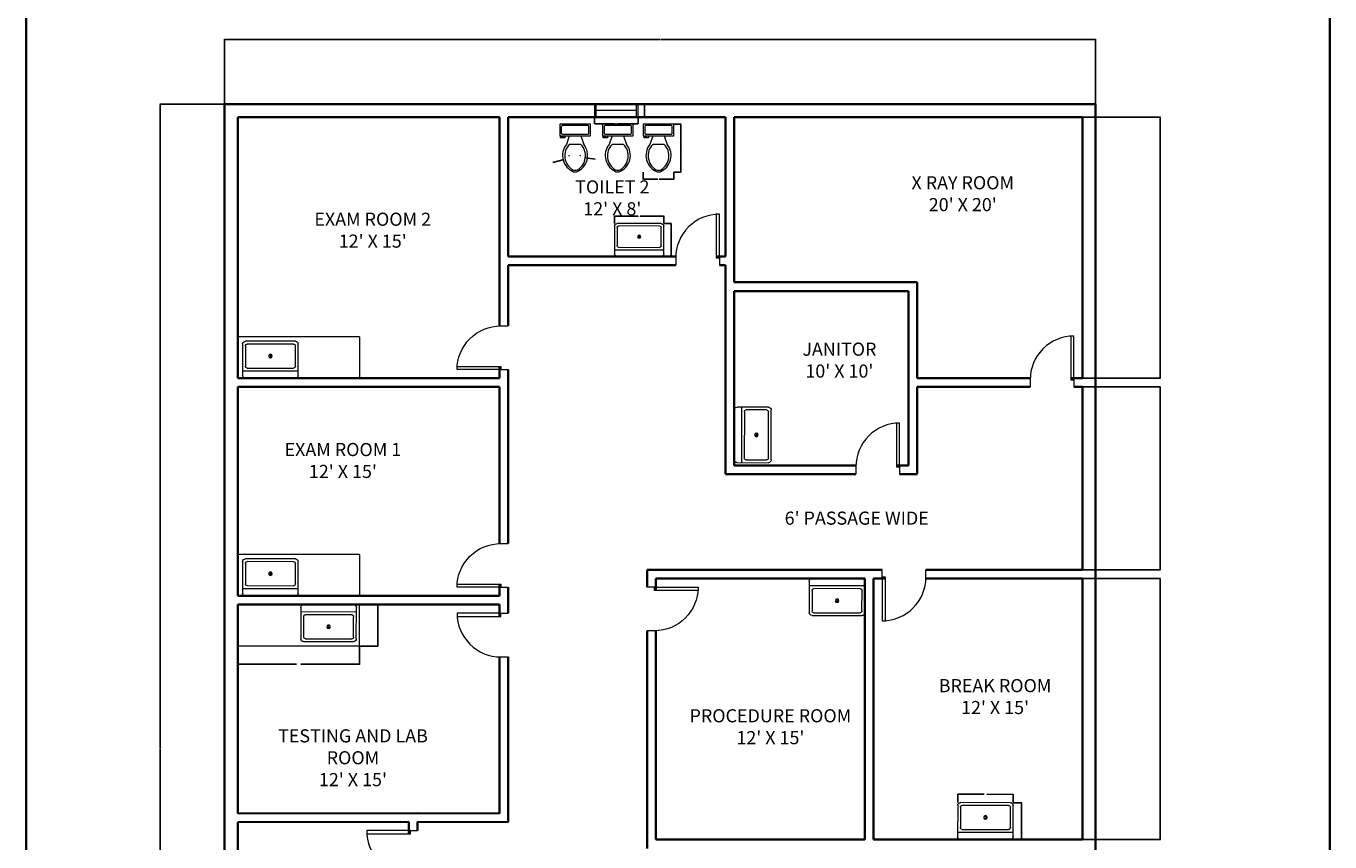
# Model space of a CAD drawing. Units: inches. Extents: x 7245 to 8143, y 15548 to 17244.
# Tile 4 of 5: x 7245 to 8143, y 16334 to 16896. Entities that reach past the tile are written whole.
import ezdxf

# ---------------------------------------------------------------- set-up
doc = ezdxf.new("R2010")
doc.units = ezdxf.units.IN
for name, color, linetype, lineweight in [('A-ANNO-DIMS', 2, 'Continuous', 18), ('A-ANNO-TTLB', 7, 'Continuous', 35), ('A-AREA-IDEN', 7, 'Continuous', 18), ('A-DOOR', 3, 'Continuous', 18), ('A-FLOR-CASE', 9, 'Continuous', 20), ('A-FLOR-FIXT', 9, 'Continuous', 18), ('A-GLAZ', 4, 'Continuous', 18), ('A-WALL', 7, 'Continuous', 35)]:
    doc.layers.add(name, color=color, linetype=linetype, lineweight=lineweight)
doc.styles.get("Standard").update_dxf_attribs({"font": 'arial.ttf'})
doc.dimstyles.get("Standard").update_dxf_attribs({"dimtxt": 0.18, "dimasz": 0.18, "dimexe": 0.18, "dimexo": 0.0625, "dimgap": 0.09, "dimtad": 0, "dimtih": 1, "dimtoh": 1, "dimdec": 4, "dimzin": 0, "dimdsep": 46, "dimtxsty": 'Standard', "dimcen": 0.09, "dimadec": 0, "dimazin": 0, "dimtfac": 1, "dimtdec": 4, "dimtofl": 0, "dimtmove": 0, "dimatfit": 3, "dimfxl": 1, "dimtolj": 1, "dimtzin": 0, "dimarcsym": 0})

# ---------------------------------------------------------------- blocks, each defined once
blk = doc.blocks.new('Sink-single - 30 in top')
blk.add_line((-15, -3.999996), (15, -3.999996))
for points in [[(-13.5, 0), (13.5, 0)], [(-15, -18.499996), (-15, -1.5)], [(-13.5, -17.499996), (-13.5, -6.499996)], [(-12.5, -5.499996), (12.5, -5.499996)], [(13.5, -6.499996), (13.5, -17.499996)], [(15, -1.5), (15, -18.499996)], [(13.5, -19.999996), (-13.5, -19.999996)], [(12.5, -18.499996), (-12.5, -18.499996)]]:
    blk.add_lwpolyline(points)
for radius in [1, 0.5]:
    blk.add_circle((0, -11.999996), radius)
for centre, radius, start, end in [((-13.5, -1.5), 1.5, 90, 180), ((-12.5, -6.499996), 1, 90, 180), ((12.5, -6.499996), 1, 0, 90), ((13.5, -1.5), 1.5, 0, 90), ((-13.5, -18.499996), 1.5, 180, 270), ((-12.5, -17.499996), 1, 180, 270), ((12.5, -17.499996), 1, 270, 0), ((13.5, -18.499996), 1.5, 270, 0)]:
    blk.add_arc(centre, radius, start, end)
blk = doc.blocks.new('*U9')
for p, q in [((0, 0), (0, 100)), ((600, 0), (600, 100))]:
    blk.add_line(p, q)
blk.add_lwpolyline([(0, 0), (0, -600), (43.75, -600), (43.75, 0)], close=True)
blk.add_arc((0, 0), 600, 270, 0)
blk = doc.blocks.new('Toilet - top')
for p, q in [((-10, -8.5), (-8, -8.5)), ((-10, -9.5), (-10, -8.5)), ((-8, -8.5), (-8, -8)), ((-7, -8), (-7, -9.5)), ((-4, -8), (-6, -14)), ((4, -8), (6, -14)), ((9.5, -6), (9.5, -2)), ((-7, -9.5), (-10, -9.5)), ((4, -14), (-4, -14))]:
    blk.add_line(p, q)
blk.add_lwpolyline([(10.5, -8), (10.5, 0), (-10.5, 0), (-10.5, -8)], close=True)
for points in [[(-9.5, -2), (-9.5, -6)], [(8.5, -1), (-8.5, -1)], [(-8.5, -7), (8.5, -7)]]:
    blk.add_lwpolyline(points)
for centre, radius, start, end in [((-8.62, -1.88), 0.884, 81.8699, 188.1301), ((-8.62, -6.12), 0.884, 171.8699, 278.1301), ((8.62, -1.88), 0.884, 351.8699, 98.1301), ((8.62, -6.12), 0.884, 261.8699, 8.1301), ((3.52, -21.58), 12.17, 141.46911, 247.97143), ((4.2, -21.82), 11.33, 136.36773, 238.94682), ((-3.52, -21.58), 12.17, 292.02843, 38.53071), ((-4.2, -21.82), 11.33, 301.05301, 43.63209), ((0, -27.88), 4, 245.73182, 294.26817), ((0, -29), 4, 254.86053, 285.13947)]:
    blk.add_arc(centre, radius, start, end)
blk = doc.blocks.new('WINDOW-30IN-PLAN')
for p, q in [((30, 9), (0, 9)), ((0, 9), (0, 0)), ((1, 9), (1, 0)), ((29, 0), (29, 9)), ((30, 0), (30, 9)), ((29, 4.5), (1, 4.5)), ((0, 0), (30, 0))]:
    blk.add_line(p, q)
blk = doc.blocks.new('SINK-COUNTER-84IN')
for q in [(84, 28.58), (0, 0)]:
    blk.add_line((84, 0), q)
blk = doc.blocks.new('*D20')
at = {"layer": 'A-ANNO-DIMS', "color": 0, "lineweight": -2, "transparency": 16777216}
for p, q in [((7887.06, 16360.81), (7887.08, 16366.67)), ((7887.26, 16366.49), (7905.26, 16366.45)), ((7925.14, 16366.4), (7907.13, 16366.44)), ((7925.31, 16360.73), (7925.32, 16366.58))]:
    blk.add_line(p, q, dxfattribs=at)
at = {"layer": 'A-ANNO-DIMS', "color": 0, "transparency": 16777216}
for points in [[(7887.26, 16366.52), (7887.26, 16366.46), (7887.08, 16366.49)], [(7925.14, 16366.43), (7925.14, 16366.37), (7925.32, 16366.4)]]:
    blk.add_solid(points, dxfattribs=at)
at = {"layer": 'Defpoints', "color": 0, "transparency": 16777216}
for p in [(7925.32, 16366.4), (7887.06, 16360.75), (7925.31, 16360.67)]:
    blk.add_point(p, dxfattribs=at)
at = {"layer": 'A-ANNO-DIMS', "color": 0, "transparency": 16777216, "insert": (7906.2, 16366.44), "char_height": 0.18, "attachment_point": 5}
blk.add_mtext('\\A1;BASIN 38 TYP.', dxfattribs=at)
blk = doc.blocks.new('*D21')
at = {"layer": 'A-ANNO-DIMS', "color": 0, "lineweight": -2, "transparency": 16777216}
for p, q in [((7925.37, 16360.67), (7931.22, 16360.65)), ((7931.04, 16360.48), (7931.02, 16348.09)), ((7930.99, 16335.34), (7931.01, 16347.73)), ((7925.31, 16335.17), (7931.17, 16335.16))]:
    blk.add_line(p, q, dxfattribs=at)
at = {"layer": 'A-ANNO-DIMS', "color": 0, "transparency": 16777216}
for points in [[(7931.01, 16360.48), (7931.07, 16360.48), (7931.04, 16360.66)], [(7930.96, 16335.34), (7931.02, 16335.34), (7930.99, 16335.16)]]:
    blk.add_solid(points, dxfattribs=at)
at = {"layer": 'Defpoints', "color": 0, "transparency": 16777216}
for p in [(7925.31, 16360.67), (7925.25, 16335.17), (7930.99, 16335.16)]:
    blk.add_point(p, dxfattribs=at)
at = {"layer": 'A-ANNO-DIMS', "color": 0, "transparency": 16777216, "insert": (7931.02, 16347.91), "char_height": 0.18, "attachment_point": 5}
blk.add_mtext('\\A1;25 TYP.', dxfattribs=at)
blk = doc.blocks.new('*D22')
at = {"layer": 'A-ANNO-DIMS', "color": 0, "lineweight": -2, "transparency": 16777216}
for p, q in [((7650.71, 16759.93), (7650.72, 16765.13)), ((7650.9, 16764.95), (7667.03, 16764.92)), ((7684.42, 16764.88), (7668.29, 16764.91)), ((7684.59, 16759.86), (7684.6, 16765.06))]:
    blk.add_line(p, q, dxfattribs=at)
at = {"layer": 'A-ANNO-DIMS', "color": 0, "transparency": 16777216}
for points in [[(7650.9, 16764.98), (7650.9, 16764.92), (7650.72, 16764.95)], [(7684.42, 16764.91), (7684.42, 16764.85), (7684.6, 16764.88)]]:
    blk.add_solid(points, dxfattribs=at)
at = {"layer": 'Defpoints', "color": 0, "transparency": 16777216}
for p in [(7684.6, 16764.88), (7650.71, 16759.87), (7684.59, 16759.8)]:
    blk.add_point(p, dxfattribs=at)
at = {"layer": 'A-ANNO-DIMS', "color": 0, "transparency": 16777216, "insert": (7667.66, 16764.92), "char_height": 0.18, "attachment_point": 5}
blk.add_mtext('\\A1;BASIN 34', dxfattribs=at)
blk = doc.blocks.new('*D23')
at = {"layer": 'A-ANNO-DIMS', "color": 0, "lineweight": -2, "transparency": 16777216}
for p, q in [((7684.65, 16759.8), (7689.85, 16759.79)), ((7689.67, 16759.61), (7689.65, 16748.67)), ((7689.62, 16737.38), (7689.65, 16748.31)), ((7684.6, 16737.21), (7689.8, 16737.2))]:
    blk.add_line(p, q, dxfattribs=at)
at = {"layer": 'A-ANNO-DIMS', "color": 0, "transparency": 16777216}
for points in [[(7689.64, 16759.61), (7689.7, 16759.61), (7689.67, 16759.79)], [(7689.59, 16737.38), (7689.65, 16737.38), (7689.62, 16737.2)]]:
    blk.add_solid(points, dxfattribs=at)
at = {"layer": 'Defpoints', "color": 0, "transparency": 16777216}
for p in [(7684.59, 16759.8), (7684.54, 16737.21), (7689.62, 16737.2)]:
    blk.add_point(p, dxfattribs=at)
at = {"layer": 'A-ANNO-DIMS', "color": 0, "transparency": 16777216, "insert": (7689.65, 16748.49), "char_height": 0.18, "attachment_point": 5}
blk.add_mtext('\\A1;23', dxfattribs=at)
blk = doc.blocks.new('*D30')
at = {"layer": 'A-ANNO-DIMS', "color": 0, "lineweight": -2, "transparency": 16777216}
for p, q in [((7691.53, 16828.41), (7696.61, 16828.41)), ((7696.43, 16828.23), (7696.43, 16812.07)), ((7696.43, 16795.54), (7696.43, 16811.7)), ((7691.53, 16795.36), (7696.61, 16795.36))]:
    blk.add_line(p, q, dxfattribs=at)
at = {"layer": 'A-ANNO-DIMS', "color": 0, "transparency": 16777216}
for points in [[(7696.4, 16828.23), (7696.46, 16828.23), (7696.43, 16828.41)], [(7696.4, 16795.54), (7696.46, 16795.54), (7696.43, 16795.36)]]:
    blk.add_solid(points, dxfattribs=at)
at = {"layer": 'Defpoints', "color": 0, "transparency": 16777216}
for p in [(7691.47, 16828.41), (7696.43, 16828.41), (7691.47, 16795.36)]:
    blk.add_point(p, dxfattribs=at)
at = {"layer": 'A-ANNO-DIMS', "color": 0, "transparency": 16777216, "insert": (7696.43, 16811.89), "char_height": 0.18, "attachment_point": 5}
blk.add_mtext('\\A1;WC 33 TYP.', dxfattribs=at)
blk = doc.blocks.new('*D31')
at = {"layer": 'A-ANNO-DIMS', "color": 0, "lineweight": -2, "transparency": 16777216}
for p, q in [((7670.47, 16795.3), (7670.47, 16790.23)), ((7670.65, 16790.41), (7680.44, 16790.41)), ((7691.29, 16790.41), (7681.5, 16790.41)), ((7691.47, 16795.3), (7691.47, 16790.23))]:
    blk.add_line(p, q, dxfattribs=at)
at = {"layer": 'A-ANNO-DIMS', "color": 0, "transparency": 16777216}
for points in [[(7670.65, 16790.44), (7670.65, 16790.38), (7670.47, 16790.41)], [(7691.29, 16790.44), (7691.29, 16790.38), (7691.47, 16790.41)]]:
    blk.add_solid(points, dxfattribs=at)
at = {"layer": 'Defpoints', "color": 0, "transparency": 16777216}
for p in [(7670.47, 16795.36), (7691.47, 16795.36), (7691.47, 16790.41)]:
    blk.add_point(p, dxfattribs=at)
at = {"layer": 'A-ANNO-DIMS', "color": 0, "transparency": 16777216, "insert": (7680.97, 16790.41), "char_height": 0.18, "attachment_point": 5}
blk.add_mtext('\\A1;21 TYP.', dxfattribs=at)
blk = doc.blocks.new('*D32')
at = {"layer": 'A-ANNO-DIMS', "color": 0, "lineweight": -2, "transparency": 16777216}
for p, q in [((7391.08, 16468.57), (7391.08, 16455.85)), ((7475.08, 16468.57), (7475.08, 16455.85)), ((7391.26, 16456.03), (7431.57, 16456.03)), ((7474.9, 16456.03), (7434.6, 16456.03))]:
    blk.add_line(p, q, dxfattribs=at)
at = {"layer": 'A-ANNO-DIMS', "color": 0, "transparency": 16777216}
for points in [[(7391.26, 16456.06), (7391.26, 16456), (7391.08, 16456.03)], [(7474.9, 16456.06), (7474.9, 16456), (7475.08, 16456.03)]]:
    blk.add_solid(points, dxfattribs=at)
at = {"layer": 'Defpoints', "color": 0, "transparency": 16777216}
for p in [(7391.08, 16468.63), (7475.08, 16468.63), (7475.08, 16456.03)]:
    blk.add_point(p, dxfattribs=at)
at = {"layer": 'A-ANNO-DIMS', "color": 0, "transparency": 16777216, "insert": (7433.08, 16456.03), "char_height": 0.18, "attachment_point": 5}
blk.add_mtext('\\A1;SINK COUNTER 84 TYP.', dxfattribs=at)
blk = doc.blocks.new('*D33')
at = {"layer": 'A-ANNO-DIMS', "color": 0, "lineweight": -2, "transparency": 16777216}
for p, q in [((7475.15, 16497.21), (7487.86, 16497.21)), ((7487.68, 16497.03), (7487.68, 16483.11)), ((7487.68, 16468.81), (7487.68, 16482.74)), ((7475.15, 16468.63), (7487.86, 16468.63))]:
    blk.add_line(p, q, dxfattribs=at)
at = {"layer": 'A-ANNO-DIMS', "color": 0, "transparency": 16777216}
for points in [[(7487.65, 16497.03), (7487.71, 16497.03), (7487.68, 16497.21)], [(7487.65, 16468.81), (7487.71, 16468.81), (7487.68, 16468.63)]]:
    blk.add_solid(points, dxfattribs=at)
at = {"layer": 'Defpoints', "color": 0, "transparency": 16777216}
for p in [(7475.08, 16497.21), (7487.68, 16497.21), (7475.08, 16468.63)]:
    blk.add_point(p, dxfattribs=at)
at = {"layer": 'A-ANNO-DIMS', "color": 0, "transparency": 16777216, "insert": (7487.68, 16482.92), "char_height": 0.18, "attachment_point": 5}
blk.add_mtext('\\A1;29 TYP.', dxfattribs=at)
blk = doc.blocks.new('*D36')
at = {"layer": 'A-ANNO-DIMS', "color": 0, "lineweight": -2, "transparency": 16777216}
for p, q in [((7636.84, 16833.13), (7636.84, 16828.51)), ((7666.84, 16833.13), (7666.84, 16828.51)), ((7637.02, 16828.69), (7650.72, 16828.69)), ((7666.66, 16828.69), (7652.96, 16828.69))]:
    blk.add_line(p, q, dxfattribs=at)
at = {"layer": 'A-ANNO-DIMS', "color": 0, "transparency": 16777216}
for points in [[(7637.02, 16828.72), (7637.02, 16828.66), (7636.84, 16828.69)], [(7666.66, 16828.72), (7666.66, 16828.66), (7666.84, 16828.69)]]:
    blk.add_solid(points, dxfattribs=at)
at = {"layer": 'Defpoints', "color": 0, "transparency": 16777216}
for p in [(7636.84, 16833.19), (7666.84, 16833.19), (7666.84, 16828.69)]:
    blk.add_point(p, dxfattribs=at)
at = {"layer": 'A-ANNO-DIMS', "color": 0, "transparency": 16777216, "insert": (7651.84, 16828.69), "char_height": 0.18, "attachment_point": 5}
blk.add_mtext('\\A1;WINDOW 30 TYP.', dxfattribs=at)
blk = doc.blocks.new('*D37')
at = {"layer": 'A-ANNO-DIMS', "color": 0, "lineweight": -2, "transparency": 16777216}
for p, q in [((7666.91, 16842.19), (7671.52, 16842.19)), ((7671.34, 16842.01), (7671.34, 16837.87)), ((7666.91, 16833.19), (7671.52, 16833.19)), ((7671.34, 16833.37), (7671.34, 16837.51))]:
    blk.add_line(p, q, dxfattribs=at)
at = {"layer": 'A-ANNO-DIMS', "color": 0, "transparency": 16777216}
for points in [[(7671.31, 16842.01), (7671.37, 16842.01), (7671.34, 16842.19)], [(7671.31, 16833.37), (7671.37, 16833.37), (7671.34, 16833.19)]]:
    blk.add_solid(points, dxfattribs=at)
at = {"layer": 'Defpoints', "color": 0, "transparency": 16777216}
for p in [(7666.84, 16842.19), (7671.34, 16842.19), (7666.84, 16833.19)]:
    blk.add_point(p, dxfattribs=at)
at = {"layer": 'A-ANNO-DIMS', "color": 0, "transparency": 16777216, "insert": (7671.34, 16837.69), "char_height": 0.18, "attachment_point": 5}
blk.add_mtext('\\A1;9 TYP.', dxfattribs=at)
blk = doc.blocks.new('*D42')
at = {"layer": 'A-ANNO-DIMS', "color": 0, "lineweight": -2, "transparency": 16777216}
for p, q in [((7382.08, 16842.25), (7382.08, 16886.87)), ((7382.26, 16886.69), (7681.79, 16886.69)), ((7981.9, 16886.69), (7682.37, 16886.69)), ((7982.08, 16842.25), (7982.08, 16886.87))]:
    blk.add_line(p, q, dxfattribs=at)
at = {"layer": 'A-ANNO-DIMS', "color": 0, "transparency": 16777216}
for points in [[(7382.26, 16886.72), (7382.26, 16886.66), (7382.08, 16886.69)], [(7981.9, 16886.72), (7981.9, 16886.66), (7982.08, 16886.69)]]:
    blk.add_solid(points, dxfattribs=at)
at = {"layer": 'Defpoints', "color": 0, "transparency": 16777216}
for p in [(7982.08, 16886.69), (7382.08, 16842.19), (7982.08, 16842.19)]:
    blk.add_point(p, dxfattribs=at)
at = {"layer": 'A-ANNO-DIMS', "color": 0, "transparency": 16777216, "insert": (7682.08, 16886.69), "char_height": 0.18, "attachment_point": 5}
blk.add_mtext('\\A1;600', dxfattribs=at)
blk = doc.blocks.new('*D43')
at = {"layer": 'A-ANNO-DIMS', "color": 0, "lineweight": -2, "transparency": 16777216}
for p, q in [((7382.02, 16842.19), (7337.4, 16842.19)), ((7337.58, 16842.01), (7337.58, 16398.37)), ((7337.58, 15954.37), (7337.58, 16398.01)), ((7382.02, 15954.19), (7337.4, 15954.19))]:
    blk.add_line(p, q, dxfattribs=at)
at = {"layer": 'A-ANNO-DIMS', "color": 0, "transparency": 16777216}
for points in [[(7337.55, 16842.01), (7337.61, 16842.01), (7337.58, 16842.19)], [(7337.55, 15954.37), (7337.61, 15954.37), (7337.58, 15954.19)]]:
    blk.add_solid(points, dxfattribs=at)
at = {"layer": 'Defpoints', "color": 0, "transparency": 16777216}
for p in [(7337.58, 16842.19), (7382.08, 16842.19), (7382.08, 15954.19)]:
    blk.add_point(p, dxfattribs=at)
at = {"layer": 'A-ANNO-DIMS', "color": 0, "transparency": 16777216, "insert": (7337.58, 16398.19), "char_height": 0.18, "attachment_point": 5}
blk.add_mtext('\\A1;888', dxfattribs=at)
blk = doc.blocks.new('*D50')
at = {"layer": 'A-ANNO-DIMS', "color": 0, "lineweight": -2, "transparency": 16777216}
for p, q in [((7973.15, 16515.19), (8026.76, 16515.19)), ((8026.58, 16515.01), (8026.58, 16425.37)), ((8026.58, 16335.37), (8026.58, 16425.01)), ((7973.15, 16335.19), (8026.76, 16335.19))]:
    blk.add_line(p, q, dxfattribs=at)
at = {"layer": 'A-ANNO-DIMS', "color": 0, "transparency": 16777216}
for points in [[(8026.55, 16515.01), (8026.61, 16515.01), (8026.58, 16515.19)], [(8026.55, 16335.37), (8026.61, 16335.37), (8026.58, 16335.19)]]:
    blk.add_solid(points, dxfattribs=at)
at = {"layer": 'Defpoints', "color": 0, "transparency": 16777216}
for p in [(7973.08, 16515.19), (8026.58, 16515.19), (7973.08, 16335.19)]:
    blk.add_point(p, dxfattribs=at)
at = {"layer": 'A-ANNO-DIMS', "color": 0, "transparency": 16777216, "insert": (8026.58, 16425.19), "char_height": 0.18, "attachment_point": 5}
blk.add_mtext('\\A1;180', dxfattribs=at)
blk = doc.blocks.new('*D51')
at = {"layer": 'A-ANNO-DIMS', "color": 0, "lineweight": -2, "transparency": 16777216}
for p, q in [((7973.15, 16647.19), (8026.76, 16647.19)), ((8026.58, 16647.01), (8026.58, 16584.37)), ((8026.58, 16521.37), (8026.58, 16584.01)), ((7973.15, 16521.19), (8026.76, 16521.19))]:
    blk.add_line(p, q, dxfattribs=at)
at = {"layer": 'A-ANNO-DIMS', "color": 0, "transparency": 16777216}
for points in [[(8026.55, 16647.01), (8026.61, 16647.01), (8026.58, 16647.19)], [(8026.55, 16521.37), (8026.61, 16521.37), (8026.58, 16521.19)]]:
    blk.add_solid(points, dxfattribs=at)
at = {"layer": 'Defpoints', "color": 0, "transparency": 16777216}
for p in [(7973.08, 16647.19), (8026.58, 16647.19), (7973.08, 16521.19)]:
    blk.add_point(p, dxfattribs=at)
at = {"layer": 'A-ANNO-DIMS', "color": 0, "transparency": 16777216, "insert": (8026.58, 16584.19), "char_height": 0.18, "attachment_point": 5}
blk.add_mtext('\\A1;126', dxfattribs=at)
blk = doc.blocks.new('*D52')
at = {"layer": 'A-ANNO-DIMS', "color": 0, "lineweight": -2, "transparency": 16777216}
for p, q in [((7973.15, 16833.19), (8026.76, 16833.19)), ((8026.58, 16833.01), (8026.58, 16743.37)), ((8026.58, 16653.37), (8026.58, 16743.01)), ((7973.15, 16653.19), (8026.76, 16653.19))]:
    blk.add_line(p, q, dxfattribs=at)
at = {"layer": 'A-ANNO-DIMS', "color": 0, "transparency": 16777216}
for points in [[(8026.55, 16833.01), (8026.61, 16833.01), (8026.58, 16833.19)], [(8026.55, 16653.37), (8026.61, 16653.37), (8026.58, 16653.19)]]:
    blk.add_solid(points, dxfattribs=at)
at = {"layer": 'Defpoints', "color": 0, "transparency": 16777216}
for p in [(7973.08, 16833.19), (8026.58, 16833.19), (7973.08, 16653.19)]:
    blk.add_point(p, dxfattribs=at)
at = {"layer": 'A-ANNO-DIMS', "color": 0, "transparency": 16777216, "insert": (8026.58, 16743.19), "char_height": 0.18, "attachment_point": 5}
blk.add_mtext('\\A1;180', dxfattribs=at)
blk = doc.blocks.new('*D81')
at = {"layer": 'A-ANNO-DIMS', "color": 0, "lineweight": -2, "transparency": 16777216}
for p, q in [((7626.94, 16806.83), (7627.12, 16806.83)), ((7627.03, 16806.74), (7627.03, 16806.92)), ((7608.2, 16801.88), (7615.08, 16803.69))]:
    blk.add_line(p, q, dxfattribs=at)
at = {"layer": 'A-ANNO-DIMS', "color": 0, "transparency": 16777216}
blk.add_solid([(7615.08, 16803.72), (7615.09, 16803.66), (7615.26, 16803.74)], dxfattribs=at)
at = {"layer": 'Defpoints', "color": 0, "transparency": 16777216}
for p in [(7627.03, 16806.83), (7615.26, 16803.74)]:
    blk.add_point(p, dxfattribs=at)
at = {"layer": 'A-ANNO-DIMS', "color": 0, "transparency": 16777216, "insert": (7607.52, 16801.88), "char_height": 0.18, "attachment_point": 5}
blk.add_mtext('\\A1;8X R12.17', dxfattribs=at)
blk = doc.blocks.new('*D82')
at = {"layer": 'A-ANNO-DIMS', "color": 0, "lineweight": -2, "transparency": 16777216}
for p, q in [((7619.22, 16806.59), (7619.4, 16806.59)), ((7619.31, 16806.5), (7619.31, 16806.68)), ((7637.27, 16804.18), (7630.72, 16805.06))]:
    blk.add_line(p, q, dxfattribs=at)
at = {"layer": 'A-ANNO-DIMS', "color": 0, "transparency": 16777216}
blk.add_solid([(7630.72, 16805.09), (7630.71, 16805.03), (7630.54, 16805.08)], dxfattribs=at)
at = {"layer": 'Defpoints', "color": 0, "transparency": 16777216}
for p in [(7619.31, 16806.59), (7630.54, 16805.08)]:
    blk.add_point(p, dxfattribs=at)
at = {"layer": 'A-ANNO-DIMS', "color": 0, "transparency": 16777216, "insert": (7637.95, 16804.18), "char_height": 0.18, "attachment_point": 5}
blk.add_mtext('\\A1;8X R11.33', dxfattribs=at)

msp = doc.modelspace()

# ---------------------------------------------------------------- linework, layer by layer
at = {"layer": 'A-ANNO-TTLB'}
msp.add_lwpolyline([(7245.2864, 17243.9412), (8143.486, 17243.9412), (8143.486, 15548.1459), (7245.2864, 15548.1459)], close=True, dxfattribs=at)
at = {"layer": 'A-WALL'}
for p, q in [((7382.0838, 16842.1899), (7982.0838, 16842.1899)), ((7382.0838, 15954.1899), (7382.0838, 16842.1899)), ((7982.0838, 16842.1899), (7982.0838, 15954.1899)), ((7391.0838, 16833.1899), (7571.3205, 16833.1899)), ((7391.0838, 16653.1894), (7391.0838, 16833.1899)), ((7571.3205, 16689.2844), (7571.3205, 16833.1899)), ((7577.3205, 16833.1899), (7727.0838, 16833.1899)), ((7577.3205, 16833.1899), (7577.3205, 16737.1899)), ((7577.3205, 16737.1899), (7577.3205, 16833.1899)), ((7727.0838, 16833.1899), (7727.0838, 16737.1899)), ((7733.0838, 16833.1899), (7733.0838, 16719.339)), ((7733.0838, 16833.1899), (7973.0838, 16833.1899)), ((7973.0838, 16833.1899), (7973.0838, 16653.1899)), ((7577.3205, 16737.1899), (7692.8042, 16737.1899)), ((7720.7028, 16737.1899), (7727.0838, 16737.1899)), ((7577.3205, 16731.1899), (7692.7882, 16731.1899)), ((7577.3205, 16689.3004), (7577.3205, 16731.1899)), ((7722.8983, 16731.1899), (7727.0838, 16731.1899)), ((7727.0838, 16731.1899), (7727.0838, 16647.1899)), ((7733.0838, 16719.339), (7859.0838, 16719.339)), ((7859.0838, 16653.1899), (7859.0838, 16719.339)), ((7733.0838, 16713.339), (7853.0838, 16713.339)), ((7733.0838, 16713.339), (7733.0838, 16653.1899)), ((7853.0838, 16653.1899), (7853.0838, 16713.339)), ((7391.0838, 16653.1894), (7571.3205, 16653.1903)), ((7571.3205, 16653.1903), (7571.3205, 16661.3859)), ((7577.3205, 16653.1904), (7577.3205, 16659.1903)), ((7577.3205, 16653.1904), (7577.3384, 16539.3008)), ((7733.0838, 16653.1899), (7733.0838, 16593.1899)), ((7853.0838, 16653.1899), (7853.0838, 16647.1899)), ((7859.0838, 16653.1899), (7936.9897, 16653.1899)), ((7964.8882, 16653.1899), (7973.0838, 16653.1899)), ((7973.0838, 16653.1899), (7967.0838, 16653.1899)), ((7391.0838, 16503.1897), (7391.083, 16647.1897)), ((7391.0838, 16647.1894), (7571.3205, 16647.1894)), ((7391.0838, 16503.1897), (7391.0838, 16647.1894)), ((7571.3205, 16647.1894), (7571.3205, 16539.284)), ((7727.0838, 16587.1899), (7727.0838, 16647.1899)), ((7853.0838, 16593.1899), (7853.0838, 16647.1899)), ((7859.0838, 16647.1899), (7859.0838, 16593.1899)), ((7936.9736, 16647.1899), (7859.0838, 16647.1899)), ((7973.0838, 16647.1899), (7967.0838, 16647.1899)), ((7973.0838, 16647.1899), (7973.0838, 16521.1899)), ((7733.0838, 16593.1899), (7816.9897, 16593.1899)), ((7844.8882, 16593.1899), (7853.0838, 16593.1899)), ((7859.0838, 16593.1899), (7859.0838, 16587.1899)), ((7816.9736, 16587.1899), (7727.0838, 16587.1899)), ((7859.0838, 16587.1899), (7847.0838, 16587.1899)), ((7679.0838, 16521.1899), (7673.0838, 16521.1899)), ((7673.0838, 16521.1899), (7673.0838, 16509.1899)), ((7823.1503, 16521.1899), (7679.0838, 16521.1899)), ((7829.0838, 16521.1899), (7823.1503, 16521.1899)), ((7835.0838, 16521.1899), (7829.0838, 16521.1899)), ((7973.0838, 16521.1899), (7865.1939, 16521.1899)), ((7571.3205, 16511.3862), (7571.3205, 16503.1894)), ((7577.3431, 16509.1906), (7577.345, 16497.1895)), ((7679.0838, 16515.1899), (7823.1482, 16515.1384)), ((7679.0838, 16506.9944), (7679.0838, 16515.1899)), ((7823.1482, 16515.1384), (7823.0838, 16335.1899)), ((7829.0838, 16335.1899), (7829.0838, 16515.1899)), ((7829.0838, 16515.1899), (7837.2793, 16515.1899)), ((7865.1779, 16515.1899), (7973.0838, 16515.1899)), ((7973.0838, 16515.1899), (7973.0838, 16335.1899)), ((7391.0838, 16503.1897), (7571.3205, 16503.1906)), ((7577.3205, 16503.1906), (7577.3224, 16491.1897)), ((7391.0838, 16353.1899), (7391.0838, 16497.1897)), ((7391.0838, 16497.1897), (7571.3205, 16497.1897)), ((7571.3205, 16497.1897), (7571.3205, 16488.9942)), ((7673.0838, 16479.0798), (7673.0838, 16335.1899)), ((7679.0838, 16335.1899), (7679.0838, 16479.0958)), ((7571.3205, 16461.0964), (7571.3205, 16353.1897)), ((7577.3271, 16461.0796), (7577.345, 16347.1897)), ((7391.0739, 16353.1899), (7515.0229, 16353.3937)), ((7391.0838, 16347.1899), (7509.0229, 16347.3842)), ((7509.0229, 16347.3842), (7509.0229, 16339.1887)), ((7509.0229, 16347.3842), (7509.0229, 16341.3842)), ((7577.345, 16347.1897), (7515.0011, 16347.3941)), ((7571.3205, 16353.1897), (7515.0229, 16353.3941)), ((7515.0229, 16347.3941), (7515.0229, 16341.3842)), ((7391.0838, 16275.1899), (7391.0838, 16347.1899)), ((7673.0838, 16335.1899), (7673.0838, 16329.1899)), ((7823.0838, 16335.1899), (7679.0838, 16335.1899)), ((7973.0838, 16335.1899), (7829.0838, 16335.1899))]:
    msp.add_line(p, q, dxfattribs=at)

# ---------------------------------------------------------------- block references
at = {"layer": 'A-DOOR', "yscale": 0.0501835234749654, "zscale": 0.0501835234749654}
for p, xscale, rotation in [((7722.8983, 16736.2083), 0.0501835234749654, 180), ((7572.3022, 16659.1903), -0.0501835234749654, 270), ((7967.0838, 16652.2083), 0.0501835234749654, 180), ((7847.0838, 16592.2083), 0.0501835234749654, 180), ((7572.3248, 16509.1906), -0.0501835234749654, 270), ((7678.1021, 16509.1899), -0.0501835234749654, 90), ((7572.3248, 16491.1897), 0.0501835234749654, 270), ((7510.0271, 16341.3842), 0.0501835234749654, 270)]:
    msp.add_blockref('*U9', p, dxfattribs=dict(at, xscale=xscale, rotation=rotation))
at = {"layer": 'A-DOOR', "xscale": 0.0501835234749654, "yscale": 0.0501835234749654, "zscale": 0.0501835234749654}
msp.add_blockref('*U9', (7835.0838, 16516.1716), dxfattribs=at)
at = {"layer": 'A-FLOR-CASE', "extrusion": (0, 0, -1), "zscale": -1, "rotation": 180}
for p in [(-7391.0822, 16681.7226), (-7391.083, 16531.7228)]:
    msp.add_blockref('SINK-COUNTER-84IN', p, dxfattribs=at)
at = {"layer": 'A-FLOR-CASE'}
msp.add_blockref('SINK-COUNTER-84IN', (7391.083, 16468.632), dxfattribs=at)
at = {"layer": 'A-FLOR-FIXT'}
for p in [(7623.509, 16828.4096), (7652.9223, 16828.4096), (7680.9683, 16828.4096)]:
    msp.add_blockref('Toilet - top', p, dxfattribs=at)
for p, xscale, yscale, zscale, rotation in [((7667.6018, 16737.2463), -1.129358775807926, 1.129358775807926, 1.129358775807926, 179.8776118655341), ((7413.5572, 16653.2057), -1.274754422904, 1.274754422904, 1.274754422904, 179.8776118655341), ((7733.0832, 16614.1838), -1.274754422904, 1.274754422904, 1.274754422904, 89.87761186553415), ((7413.5579, 16503.2059), -1.274754422904, 1.274754422904, 1.274754422904, 179.8776118655341), ((7803.9752, 16515.163), -1.274754422904, 1.274754422904, 1.274754422904, 359.8776118655341), ((7453.7199, 16497.1822), -1.274754422904, 1.274754422904, 1.274754422904, 359.8776118655341), ((7906.1304, 16335.2131), -1.274754422904, 1.274754422904, 1.274754422904, 179.8776118655341)]:
    msp.add_blockref('Sink-single - 30 in top', p, dxfattribs=dict(at, xscale=xscale, yscale=yscale, zscale=zscale, rotation=rotation))
at = {"layer": 'A-GLAZ'}
msp.add_blockref('WINDOW-30IN-PLAN', (7636.843, 16833.19), dxfattribs=at)

# ---------------------------------------------------------------- texts
at = {"layer": 'A-AREA-IDEN', "char_height": 9.045999, "attachment_point": 1}
for s, insert in [("\\pxqc;{\\fArial|b1|i0|c0|p34;TOILET 2^J12' X 8'}", (7589.0214, 16789.6122)), ("\\pxqc;{\\fArial|b1|i0|c0|p34;X RAY ROOM^J20' X 20'}", (7830.4427, 16792.4936)), ("\\pxqc;{\\fArial|b1|i0|c0|p34;EXAM ROOM 2^J12' X 15'}", (7423.9735, 16767.3366)), ("\\pxqc;{\\fArial|b1|i0|c0|p34;JANITOR^J10' X 10'}", (7745.4389, 16677.7831)), ("\\pxqc;{\\fArial|b1|i0|c0|p34;EXAM ROOM 1^J12' X 15'}", (7403.423, 16608.5924)), ("\\pxqc;{\\fArial|b1|i0|c0|p34;6' PASSAGE WIDE}", (7757.3898, 16561.3048)), ("\\pxqc;{\\fArial|b1|i0|c0|p34;BREAK ROOM^J12' X 15'}", (7852.6851, 16445.8643)), ("\\pxqc;{\\fArial|b1|i0|c0|p34;PROCEDURE ROOM^J12' X 15'}", (7697.9264, 16425.0905)), ("\\pxqc;{\\fArial|b1|i0|c0|p34;TESTING AND LAB ROOM^J12' X 15'}", (7410.3525, 16411.2414))]:
    msp.add_mtext_dynamic_manual_height_columns(s, width=120.239684, gutter_width=18.8458, heights=[0], dxfattribs=dict(at, insert=insert))

# ---------------------------------------------------------------- dimensions: what is measured, and where the dimension line sits
at = {"layer": 'A-ANNO-DIMS'}
dim = msp.add_linear_dim(base=(7982.0838, 16886.6899), p1=(7382.0838, 16842.1899), p2=(7982.0838, 16842.1899), dimstyle='Standard', override={"dimdec": 0, "dimlfac": 1, "dimrnd": 0, "dimzin": 0, "dimdsep": 46, "dimlunit": 2}, dxfattribs=at)
dim.commit()
dim.dimension.update_dxf_attribs({"geometry": '*D42', "text_midpoint": (7682.0838, 16886.6899)})
for base, p1, p2, angle, picture, middle in [((7337.5838, 16842.1899), (7382.0838, 15954.1899), (7382.0838, 16842.1899), 90, '*D43', (7337.5838, 16398.1899)), ((8026.5838, 16833.1899), (7973.0838, 16653.1899), (7973.0838, 16833.1899), 90, '*D52', (8026.5838, 16743.1899)), ((7689.6242, 16737.1993), (7684.5904, 16759.7973), (7684.5421, 16737.2102), 269.8776119, '*D23', (7689.6484, 16748.4929)), ((8026.5838, 16647.1899), (7973.0838, 16521.1899), (7973.0838, 16647.1899), 90, '*D51', (8026.5838, 16584.1899)), ((8026.5838, 16515.1899), (7973.0838, 16335.1899), (7973.0838, 16515.1899), 90, '*D50', (8026.5838, 16425.1899))]:
    dim = msp.add_linear_dim(base=base, p1=p1, p2=p2, angle=angle, dimstyle='Standard', override={"dimdec": 0, "dimlfac": 1, "dimrnd": 0, "dimzin": 0, "dimdsep": 46, "dimlunit": 2}, dxfattribs=at)
    dim.commit()
    dim.dimension.update_dxf_attribs({"geometry": picture, "text_midpoint": middle})
for base, p1, p2, angle, text, picture, middle in [((7671.3433, 16842.1899), (7666.8433, 16833.1899), (7666.8433, 16842.1899), 90, '<> TYP.', '*D37', (7671.3433, 16837.6899)), ((7696.4252, 16828.4096), (7691.4683, 16795.3634), (7691.4683, 16828.4096), 90, 'WC <> TYP.', '*D30', (7696.4252, 16811.8865)), ((7684.6012, 16764.8794), (7650.7097, 16759.8697), (7684.5904, 16759.7973), 359.8776119, 'BASIN <>', '*D22', (7667.6609, 16764.9156)), ((7487.6834, 16497.2146), (7475.0834, 16468.6325), (7475.0834, 16497.2146), 90, '<> TYP.', '*D33', (7487.6834, 16482.9236)), ((7925.3184, 16366.4037), (7887.0636, 16360.749), (7925.3061, 16360.6673), 359.8776119, 'BASIN <> TYP.', '*D20', (7906.1971, 16366.4446)), ((7930.988, 16335.1601), (7925.3061, 16360.6673), (7925.2516, 16335.1723), 269.8776119, '<> TYP.', '*D21', (7931.0153, 16347.9076))]:
    dim = msp.add_linear_dim(base=base, p1=p1, p2=p2, angle=angle, text=text, dimstyle='Standard', override={"dimdec": 0, "dimlfac": 1, "dimrnd": 0, "dimzin": 0, "dimdsep": 46, "dimlunit": 2}, dxfattribs=at)
    dim.commit()
    dim.dimension.update_dxf_attribs({"geometry": picture, "text_midpoint": middle})
for base, p1, p2, text, picture, middle in [((7666.8433, 16828.6899), (7636.8433, 16833.1899), (7666.8433, 16833.1899), 'WINDOW <> TYP.', '*D36', (7651.8433, 16828.6899)), ((7691.4683, 16790.4065), (7670.4683, 16795.3634), (7691.4683, 16795.3634), '<> TYP.', '*D31', (7680.9683, 16790.4065)), ((7475.0834, 16456.0325), (7391.0834, 16468.6325), (7475.0834, 16468.6325), 'SINK COUNTER <> TYP.', '*D32', (7433.0834, 16456.0325))]:
    dim = msp.add_linear_dim(base=base, p1=p1, p2=p2, text=text, dimstyle='Standard', override={"dimdec": 0, "dimlfac": 1, "dimrnd": 0, "dimzin": 0, "dimdsep": 46, "dimlunit": 2}, dxfattribs=at)
    dim.commit()
    dim.dimension.update_dxf_attribs({"geometry": picture, "text_midpoint": middle})
for center, mpoint, picture, middle in [((7627.0285, 16806.8291), (7615.2589, 16803.737), '*D81', (7608.1972, 16801.8817)), ((7619.3091, 16806.5922), (7630.5373, 16805.083), '*D82', (7637.2742, 16804.1774))]:
    dim = msp.add_radius_dim(center=center, mpoint=mpoint, text='8X <>', dimstyle='Standard', override={"dimdec": 2, "dimlfac": 1, "dimrnd": 0, "dimzin": 0, "dimdsep": 46, "dimlunit": 2}, dxfattribs=at)
    dim.commit()
    dim.dimension.update_dxf_attribs({"geometry": picture, "text_midpoint": middle, "dimtype": 164})

doc.saveas('drawing.dxf')
